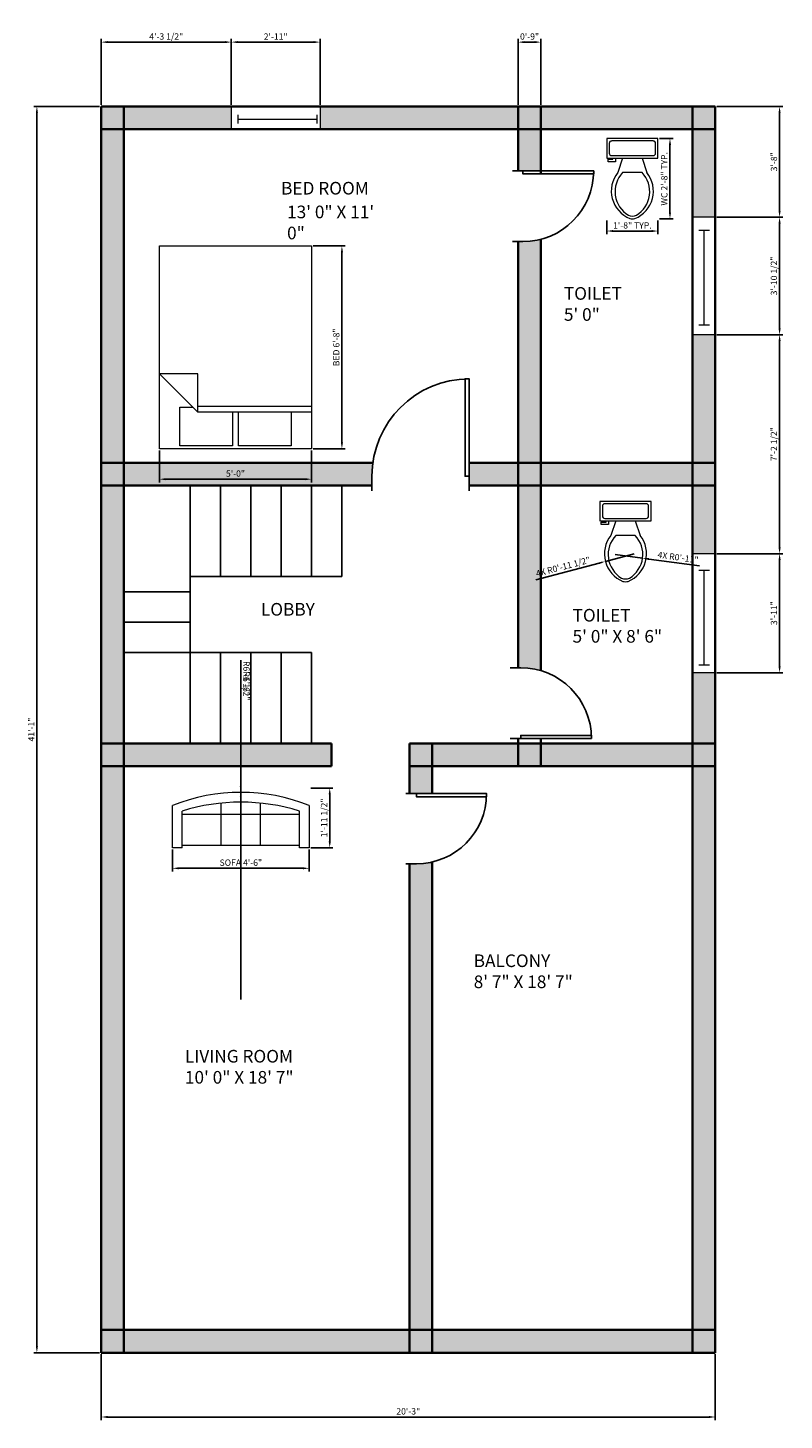
# Model space of a CAD drawing. Units: millimetres. Extents: x 2602 to 3574, y 848 to 1501.
# Tile 3 of 3: x 3274 to 3574, y 872 to 1423. Entities that reach past the tile are written whole.
import ezdxf

# ---------------------------------------------------------------- set-up
doc = ezdxf.new("R2010")
doc.units = ezdxf.units.MM
for name, color, linetype, lineweight in [('A-ANNO-DIMS', 170, 'Continuous', 18), ('A-AREA-IDEN', 200, 'Continuous', 18), ('A-FLOR-FIXT', 90, 'Continuous', 18), ('A-WALL-PATT', 140, 'Continuous', 13), ('doors', 10, 'Continuous', 25), ('furniture', 90, 'Continuous', 18), ('STAIRCASE', 30, 'Continuous', 25), ('walls', 140, 'Continuous', 35), ('windows', 40, 'Continuous', 18)]:
    doc.layers.add(name, color=color, linetype=linetype, lineweight=lineweight)
doc.styles.get("Standard").update_dxf_attribs({"font": 'arial.ttf'})
doc.dimstyles.new('ISO-25', dxfattribs={"dimtxt": 2.5, "dimasz": 2.5, "dimexe": 1.25, "dimexo": 0.625, "dimtad": 1, "dimdec": 0, "dimlunit": 3, "dimtxsty": 'Standard', "dimcen": 2.5, "dimadec": 0, "dimazin": 0, "dimtfac": 1, "dimtdec": 0, "dimtmove": 0, "dimatfit": 3, "dimfxl": 1, "dimarcsym": 0})

# ---------------------------------------------------------------- blocks, each defined once
blk = doc.blocks.new('*U2')
for p, q in [((0, 0), (0, -6)), ((40, 0), (40, -6))]:
    blk.add_line(p, q)
blk.add_lwpolyline([(0, 0), (0, 40), (1.75, 40), (1.75, 0)], close=True)
blk.add_arc((0, 0), 40, 0, 90)
blk = doc.blocks.new('*U23')
for p, q in [((0, 4), (0, 0)), ((0, 2), (36, 2)), ((36, 4), (36, 0))]:
    blk.add_line(p, q)
blk = doc.blocks.new('*U24')
for p, q in [((0, 4), (0, 0)), ((0, 2), (36, 2)), ((36, 4), (36, 0))]:
    blk.add_line(p, q)
blk = doc.blocks.new('Bed - Queen')
for p, q in [((0, -80.00003), (0, 0)), ((0, 0), (59.99999, 0)), ((59.99999, 0), (59.99999, -80.00003)), ((7.99999, -1.2), (28.79998, -1.2)), ((7.99999, -14.4), (7.99999, -1.2)), ((28.79998, -1.2), (28.79998, -14.4)), ((31.19999, -1.2), (51.99999, -1.2)), ((31.19999, -14.4), (31.19999, -1.2)), ((51.99999, -1.2), (51.99999, -16.4)), ((0, -14.4), (44.8, -14.4)), ((59.99999, -29.6), (44.8, -14.4)), ((44.8, -14.4), (44.8, -29.6)), ((51.99999, -16.4), (46.79936, -16.4)), ((44.8, -16.8), (0, -16.8)), ((44.8, -29.6), (59.99999, -29.6)), ((59.99999, -80.00003), (0, -80.00003))]:
    blk.add_line(p, q)
blk = doc.blocks.new('Sofa - Roundback 7 ft.')
for p, q in [((-12.00002, -32.4421), (-12.00003, -6.5971)), ((11.99997, -32.4421), (11.99998, -6.5971)), ((-36.000027, -34), (-36.000027, -11.4696)), ((-35.999844, -13.3819), (35.9998, -13.3819)), ((35.99998, -34), (35.99998, -11.4696)), ((-36.000027, -32.4421), (35.99998, -32.4421))]:
    blk.add_line(p, q)
for points in [[(-36.000027, -34), (-42.000027, -34), (-42.000027, -8)], [(41.99998, -8), (41.99998, -34), (35.99998, -34)]]:
    blk.add_lwpolyline(points)
for centre, radius, start, end in [((0, -114.25), 114.25, 68.43141, 111.5686), ((-0.00001, -127.1968), 121.1968, 72.72033, 107.2797)]:
    blk.add_arc(centre, radius, start, end)
blk = doc.blocks.new('Toilet - top')
for p, q in [((9.5, -6), (9.5, -2)), ((-10, -8.5), (-8, -8.5)), ((-10, -9.5), (-10, -8.5)), ((-7, -9.5), (-10, -9.5)), ((-8, -8.5), (-8, -8)), ((-7, -8), (-7, -9.5)), ((-4, -8), (-6, -14)), ((4, -8), (6, -14)), ((4, -14), (-4, -14))]:
    blk.add_line(p, q)
blk.add_lwpolyline([(10.5, -8), (10.5, 0), (-10.5, 0), (-10.5, -8)], close=True)
for points in [[(-9.5, -2), (-9.5, -6)], [(8.5, -1), (-8.5, -1)], [(-8.5, -7), (8.5, -7)]]:
    blk.add_lwpolyline(points)
for centre, radius, start, end in [((-8.62, -1.88), 0.884, 81.8699, 188.1301), ((8.62, -1.88), 0.884, 351.8699, 98.1301), ((-8.62, -6.12), 0.884, 171.8699, 278.1301), ((8.62, -6.12), 0.884, 261.8699, 8.1301), ((3.52, -21.58), 12.17, 141.4691, 247.9714), ((4.2, -21.82), 11.33, 136.3677, 238.9468), ((-3.52, -21.58), 12.17, 292.0284, 38.5307), ((-4.2, -21.82), 11.33, 301.053, 43.6321), ((0, -27.88), 4, 245.7318, 294.2682), ((0, -29), 4, 254.8605, 285.1395)]:
    blk.add_arc(centre, radius, start, end)
blk = doc.blocks.new('*D30')
at = {"layer": 'A-ANNO-DIMS', "color": 0, "lineweight": -2, "transparency": 16777216}
for p, q in [((3524.34, 1379.15), (3529.73, 1379.15)), ((3528.48, 1349.84), (3528.48, 1376.65)), ((3524.34, 1347.34), (3529.73, 1347.34))]:
    blk.add_line(p, q, dxfattribs=at)
at = {"layer": 'A-ANNO-DIMS', "color": 0, "transparency": 16777216}
for points in [[(3528.07, 1376.65), (3528.9, 1376.65), (3528.48, 1379.15)], [(3528.07, 1349.84), (3528.9, 1349.84), (3528.48, 1347.34)]]:
    blk.add_solid(points, dxfattribs=at)
at = {"layer": 'Defpoints', "color": 0, "transparency": 16777216}
for p in [(3523.71, 1379.15), (3528.48, 1379.15), (3523.71, 1347.34)]:
    blk.add_point(p, dxfattribs=at)
at = {"layer": 'A-ANNO-DIMS', "color": 0, "transparency": 16777216, "insert": (3526.56, 1363.24), "char_height": 2.5, "attachment_point": 5, "rotation": 90}
blk.add_mtext('WC 2\'-8" TYP.', dxfattribs=at)
blk = doc.blocks.new('*D31')
at = {"layer": 'A-ANNO-DIMS', "color": 0, "lineweight": -2, "transparency": 16777216}
for p, q in [((3503.49, 1346.71), (3503.49, 1341.31)), ((3523.71, 1346.71), (3523.71, 1341.31)), ((3505.99, 1342.56), (3521.21, 1342.56))]:
    blk.add_line(p, q, dxfattribs=at)
at = {"layer": 'A-ANNO-DIMS', "color": 0, "transparency": 16777216}
for points in [[(3505.99, 1342.98), (3505.99, 1342.15), (3503.49, 1342.56)], [(3521.21, 1342.98), (3521.21, 1342.15), (3523.71, 1342.56)]]:
    blk.add_solid(points, dxfattribs=at)
at = {"layer": 'Defpoints', "color": 0, "transparency": 16777216}
for p in [(3503.49, 1347.34), (3523.71, 1347.34), (3523.71, 1342.56)]:
    blk.add_point(p, dxfattribs=at)
at = {"layer": 'A-ANNO-DIMS', "color": 0, "transparency": 16777216, "insert": (3513.6, 1344.47), "char_height": 2.5, "attachment_point": 5}
blk.add_mtext('1\'-8" TYP.', dxfattribs=at)
blk = doc.blocks.new('*D34')
at = {"layer": 'A-ANNO-DIMS', "color": 0, "lineweight": -2, "transparency": 16777216}
for p, q in [((3387.25, 1336.66), (3399.91, 1336.66)), ((3398.66, 1334.16), (3398.66, 1258.93)), ((3387.25, 1256.43), (3399.91, 1256.43))]:
    blk.add_line(p, q, dxfattribs=at)
at = {"layer": 'A-ANNO-DIMS', "color": 0, "transparency": 16777216}
for points in [[(3398.25, 1334.16), (3399.08, 1334.16), (3398.66, 1336.66)], [(3398.25, 1258.93), (3399.08, 1258.93), (3398.66, 1256.43)]]:
    blk.add_solid(points, dxfattribs=at)
at = {"layer": 'Defpoints', "color": 0, "transparency": 16777216}
for p in [(3386.63, 1336.66), (3386.63, 1256.43), (3398.66, 1256.43)]:
    blk.add_point(p, dxfattribs=at)
at = {"layer": 'A-ANNO-DIMS', "color": 0, "transparency": 16777216, "insert": (3396.76, 1296.54), "char_height": 2.5, "attachment_point": 5, "rotation": 90}
blk.add_mtext('BED 6\'-8"', dxfattribs=at)
blk = doc.blocks.new('*D35')
at = {"layer": 'A-ANNO-DIMS', "color": 0, "lineweight": -2, "transparency": 16777216}
for p, q in [((3326.46, 1255.8), (3326.46, 1243.14)), ((3386.63, 1255.8), (3386.63, 1243.14)), ((3384.13, 1244.39), (3328.96, 1244.39))]:
    blk.add_line(p, q, dxfattribs=at)
at = {"layer": 'A-ANNO-DIMS', "color": 0, "transparency": 16777216}
for points in [[(3328.96, 1244.81), (3328.96, 1243.98), (3326.46, 1244.39)], [(3384.13, 1244.81), (3384.13, 1243.98), (3386.63, 1244.39)]]:
    blk.add_solid(points, dxfattribs=at)
at = {"layer": 'Defpoints', "color": 0, "transparency": 16777216}
for p in [(3326.46, 1256.43), (3386.63, 1256.43), (3326.46, 1244.39)]:
    blk.add_point(p, dxfattribs=at)
at = {"layer": 'A-ANNO-DIMS', "color": 0, "transparency": 16777216, "insert": (3356.54, 1246.29), "char_height": 2.5, "attachment_point": 5}
blk.add_mtext('5\'-0"', dxfattribs=at)
blk = doc.blocks.new('*D38')
at = {"layer": 'A-ANNO-DIMS', "color": 0, "lineweight": -2, "transparency": 16777216}
for p, q in [((3331.58, 1097.96), (3331.58, 1089.21)), ((3385.72, 1097.96), (3385.72, 1089.21)), ((3334.08, 1090.46), (3383.22, 1090.46))]:
    blk.add_line(p, q, dxfattribs=at)
at = {"layer": 'A-ANNO-DIMS', "color": 0, "transparency": 16777216}
for points in [[(3334.08, 1090.88), (3334.08, 1090.05), (3331.58, 1090.46)], [(3383.22, 1090.88), (3383.22, 1090.05), (3385.72, 1090.46)]]:
    blk.add_solid(points, dxfattribs=at)
at = {"layer": 'Defpoints', "color": 0, "transparency": 16777216}
for p in [(3331.58, 1098.59), (3385.72, 1098.59), (3385.72, 1090.46)]:
    blk.add_point(p, dxfattribs=at)
at = {"layer": 'A-ANNO-DIMS', "color": 0, "transparency": 16777216, "insert": (3358.65, 1092.38), "char_height": 2.5, "attachment_point": 5}
blk.add_mtext('SOFA 4\'-6"', dxfattribs=at)
blk = doc.blocks.new('*D39')
at = {"layer": 'A-ANNO-DIMS', "color": 0, "lineweight": -2, "transparency": 16777216}
for p, q in [((3386.34, 1122.22), (3395.09, 1122.22)), ((3393.84, 1101.09), (3393.84, 1119.72)), ((3386.34, 1098.59), (3395.09, 1098.59))]:
    blk.add_line(p, q, dxfattribs=at)
at = {"layer": 'A-ANNO-DIMS', "color": 0, "transparency": 16777216}
for points in [[(3393.42, 1119.72), (3394.26, 1119.72), (3393.84, 1122.22)], [(3393.42, 1101.09), (3394.26, 1101.09), (3393.84, 1098.59)]]:
    blk.add_solid(points, dxfattribs=at)
at = {"layer": 'Defpoints', "color": 0, "transparency": 16777216}
for p in [(3385.72, 1122.22), (3393.84, 1122.22), (3385.72, 1098.59)]:
    blk.add_point(p, dxfattribs=at)
at = {"layer": 'A-ANNO-DIMS', "color": 0, "transparency": 16777216, "insert": (3391.92, 1110.4), "char_height": 2.5, "attachment_point": 5, "rotation": 90}
blk.add_mtext('1\'-11 1/2"', dxfattribs=at)
blk = doc.blocks.new('*D48')
at = {"layer": 'A-ANNO-DIMS', "color": 0, "lineweight": -2, "transparency": 16777216}
for p, q in [((3303.41, 898.23), (3303.41, 872.15)), ((3546.41, 898.23), (3546.41, 872.15)), ((3305.91, 873.4), (3543.91, 873.4))]:
    blk.add_line(p, q, dxfattribs=at)
at = {"layer": 'A-ANNO-DIMS', "color": 0, "transparency": 16777216}
for points in [[(3305.91, 873.82), (3305.91, 872.99), (3303.41, 873.4)], [(3543.91, 873.82), (3543.91, 872.99), (3546.41, 873.4)]]:
    blk.add_solid(points, dxfattribs=at)
at = {"layer": 'Defpoints', "color": 0, "transparency": 16777216}
for p in [(3303.41, 898.85), (3546.41, 898.85), (3546.41, 873.4)]:
    blk.add_point(p, dxfattribs=at)
at = {"layer": 'A-ANNO-DIMS', "color": 0, "transparency": 16777216, "insert": (3424.91, 875.31), "char_height": 2.5, "attachment_point": 5}
blk.add_mtext('20\'-3"', dxfattribs=at)
blk = doc.blocks.new('*D49')
at = {"layer": 'A-ANNO-DIMS', "color": 0, "lineweight": -2, "transparency": 16777216}
for p, q in [((3302.78, 1391.85), (3276.71, 1391.85)), ((3277.96, 901.35), (3277.96, 1389.35)), ((3302.78, 898.85), (3276.71, 898.85))]:
    blk.add_line(p, q, dxfattribs=at)
at = {"layer": 'A-ANNO-DIMS', "color": 0, "transparency": 16777216}
for points in [[(3277.54, 1389.35), (3278.38, 1389.35), (3277.96, 1391.85)], [(3277.54, 901.35), (3278.38, 901.35), (3277.96, 898.85)]]:
    blk.add_solid(points, dxfattribs=at)
at = {"layer": 'Defpoints', "color": 0, "transparency": 16777216}
for p in [(3277.96, 1391.85), (3303.41, 1391.85), (3303.41, 898.85)]:
    blk.add_point(p, dxfattribs=at)
at = {"layer": 'A-ANNO-DIMS', "color": 0, "transparency": 16777216, "insert": (3276.08, 1145.35), "char_height": 2.5, "attachment_point": 5, "rotation": 90}
blk.add_mtext('41\'-1"', dxfattribs=at)
blk = doc.blocks.new('*D50')
at = {"layer": 'A-ANNO-DIMS', "color": 0, "lineweight": -2, "transparency": 16777216}
for p, q in [((3468.41, 1392.48), (3468.41, 1418.55)), ((3470.91, 1417.3), (3474.91, 1417.3)), ((3477.41, 1392.48), (3477.41, 1418.55))]:
    blk.add_line(p, q, dxfattribs=at)
at = {"layer": 'A-ANNO-DIMS', "color": 0, "transparency": 16777216}
for points in [[(3470.91, 1417.72), (3470.91, 1416.89), (3468.41, 1417.3)], [(3474.91, 1417.72), (3474.91, 1416.89), (3477.41, 1417.3)]]:
    blk.add_solid(points, dxfattribs=at)
at = {"layer": 'Defpoints', "color": 0, "transparency": 16777216}
for p in [(3477.41, 1417.3), (3468.41, 1391.85), (3477.41, 1391.85)]:
    blk.add_point(p, dxfattribs=at)
at = {"layer": 'A-ANNO-DIMS', "color": 0, "transparency": 16777216, "insert": (3472.91, 1419.2), "char_height": 2.5, "attachment_point": 5}
blk.add_mtext('0\'-9"', dxfattribs=at)
blk = doc.blocks.new('*D51')
at = {"layer": 'A-ANNO-DIMS', "color": 0, "lineweight": -2, "transparency": 16777216}
for p, q in [((3303.41, 1392.48), (3303.41, 1418.55)), ((3305.91, 1417.3), (3352.39, 1417.3)), ((3354.89, 1392.48), (3354.89, 1418.55))]:
    blk.add_line(p, q, dxfattribs=at)
at = {"layer": 'A-ANNO-DIMS', "color": 0, "transparency": 16777216}
for points in [[(3305.91, 1417.72), (3305.91, 1416.89), (3303.41, 1417.3)], [(3352.39, 1417.72), (3352.39, 1416.89), (3354.89, 1417.3)]]:
    blk.add_solid(points, dxfattribs=at)
at = {"layer": 'Defpoints', "color": 0, "transparency": 16777216}
for p in [(3354.89, 1417.3), (3303.41, 1391.85), (3354.89, 1391.85)]:
    blk.add_point(p, dxfattribs=at)
at = {"layer": 'A-ANNO-DIMS', "color": 0, "transparency": 16777216, "insert": (3329.15, 1419.22), "char_height": 2.5, "attachment_point": 5}
blk.add_mtext('4\'-3 1/2"', dxfattribs=at)
blk = doc.blocks.new('*D52')
at = {"layer": 'A-ANNO-DIMS', "color": 0, "lineweight": -2, "transparency": 16777216}
for p, q in [((3354.89, 1392.48), (3354.89, 1418.55)), ((3357.39, 1417.3), (3387.51, 1417.3)), ((3390.01, 1392.48), (3390.01, 1418.55))]:
    blk.add_line(p, q, dxfattribs=at)
at = {"layer": 'A-ANNO-DIMS', "color": 0, "transparency": 16777216}
for points in [[(3357.39, 1417.72), (3357.39, 1416.89), (3354.89, 1417.3)], [(3387.51, 1417.72), (3387.51, 1416.89), (3390.01, 1417.3)]]:
    blk.add_solid(points, dxfattribs=at)
at = {"layer": 'Defpoints', "color": 0, "transparency": 16777216}
for p in [(3390.01, 1417.3), (3354.89, 1391.85), (3390.01, 1391.85)]:
    blk.add_point(p, dxfattribs=at)
at = {"layer": 'A-ANNO-DIMS', "color": 0, "transparency": 16777216, "insert": (3372.45, 1419.18), "char_height": 2.5, "attachment_point": 5}
blk.add_mtext('2\'-11"', dxfattribs=at)
blk = doc.blocks.new('*D53')
at = {"layer": 'A-ANNO-DIMS', "color": 0, "lineweight": -2, "transparency": 16777216}
for p, q in [((3547.03, 1391.85), (3573.11, 1391.85)), ((3571.86, 1389.35), (3571.86, 1350.53)), ((3547.03, 1348.03), (3573.11, 1348.03))]:
    blk.add_line(p, q, dxfattribs=at)
at = {"layer": 'A-ANNO-DIMS', "color": 0, "transparency": 16777216}
for points in [[(3571.44, 1389.35), (3572.28, 1389.35), (3571.86, 1391.85)], [(3571.44, 1350.53), (3572.28, 1350.53), (3571.86, 1348.03)]]:
    blk.add_solid(points, dxfattribs=at)
at = {"layer": 'Defpoints', "color": 0, "transparency": 16777216}
for p in [(3546.41, 1391.85), (3546.41, 1348.03), (3571.86, 1348.03)]:
    blk.add_point(p, dxfattribs=at)
at = {"layer": 'A-ANNO-DIMS', "color": 0, "transparency": 16777216, "insert": (3569.96, 1369.94), "char_height": 2.5, "attachment_point": 5, "rotation": 90}
blk.add_mtext('3\'-8"', dxfattribs=at)
blk = doc.blocks.new('*D54')
at = {"layer": 'A-ANNO-DIMS', "color": 0, "lineweight": -2, "transparency": 16777216}
for p, q in [((3547.03, 1348.03), (3573.11, 1348.03)), ((3571.86, 1345.53), (3571.86, 1304.06)), ((3547.03, 1301.56), (3573.11, 1301.56))]:
    blk.add_line(p, q, dxfattribs=at)
at = {"layer": 'A-ANNO-DIMS', "color": 0, "transparency": 16777216}
for points in [[(3571.44, 1345.53), (3572.28, 1345.53), (3571.86, 1348.03)], [(3571.44, 1304.06), (3572.28, 1304.06), (3571.86, 1301.56)]]:
    blk.add_solid(points, dxfattribs=at)
at = {"layer": 'Defpoints', "color": 0, "transparency": 16777216}
for p in [(3546.41, 1348.03), (3546.41, 1301.56), (3571.86, 1301.56)]:
    blk.add_point(p, dxfattribs=at)
at = {"layer": 'A-ANNO-DIMS', "color": 0, "transparency": 16777216, "insert": (3569.94, 1324.79), "char_height": 2.5, "attachment_point": 5, "rotation": 90}
blk.add_mtext('3\'-10 1/2"', dxfattribs=at)
blk = doc.blocks.new('*D55')
at = {"layer": 'A-ANNO-DIMS', "color": 0, "lineweight": -2, "transparency": 16777216}
for p, q in [((3547.03, 1301.56), (3573.11, 1301.56)), ((3571.86, 1299.06), (3571.86, 1217.43)), ((3547.03, 1214.93), (3573.11, 1214.93))]:
    blk.add_line(p, q, dxfattribs=at)
at = {"layer": 'A-ANNO-DIMS', "color": 0, "transparency": 16777216}
for points in [[(3571.44, 1299.06), (3572.28, 1299.06), (3571.86, 1301.56)], [(3571.44, 1217.43), (3572.28, 1217.43), (3571.86, 1214.93)]]:
    blk.add_solid(points, dxfattribs=at)
at = {"layer": 'Defpoints', "color": 0, "transparency": 16777216}
for p in [(3546.41, 1301.56), (3546.41, 1214.93), (3571.86, 1214.93)]:
    blk.add_point(p, dxfattribs=at)
at = {"layer": 'A-ANNO-DIMS', "color": 0, "transparency": 16777216, "insert": (3569.94, 1258.24), "char_height": 2.5, "attachment_point": 5, "rotation": 90}
blk.add_mtext('7\'-2 1/2"', dxfattribs=at)
blk = doc.blocks.new('*D56')
at = {"layer": 'A-ANNO-DIMS', "color": 0, "lineweight": -2, "transparency": 16777216}
for p, q in [((3547.03, 1214.93), (3573.11, 1214.93)), ((3571.86, 1212.43), (3571.86, 1170.35)), ((3547.03, 1167.85), (3573.11, 1167.85))]:
    blk.add_line(p, q, dxfattribs=at)
at = {"layer": 'A-ANNO-DIMS', "color": 0, "transparency": 16777216}
for points in [[(3571.44, 1212.43), (3572.28, 1212.43), (3571.86, 1214.93)], [(3571.44, 1170.35), (3572.28, 1170.35), (3571.86, 1167.85)]]:
    blk.add_solid(points, dxfattribs=at)
at = {"layer": 'Defpoints', "color": 0, "transparency": 16777216}
for p in [(3546.41, 1214.93), (3546.41, 1167.85), (3571.86, 1167.85)]:
    blk.add_point(p, dxfattribs=at)
at = {"layer": 'A-ANNO-DIMS', "color": 0, "transparency": 16777216, "insert": (3569.96, 1191.39), "char_height": 2.5, "attachment_point": 5, "rotation": 90}
blk.add_mtext('3\'-11"', dxfattribs=at)
blk = doc.blocks.new('*D61')
at = {"layer": 'A-ANNO-DIMS', "color": 0, "lineweight": -2, "transparency": 16777216}
for p, q in [((3358.65, 1168.65), (3358.65, 1119.13)), ((3358.65, 1038.52), (3358.65, 1116.63))]:
    blk.add_line(p, q, dxfattribs=at)
at = {"layer": 'A-ANNO-DIMS', "color": 0, "transparency": 16777216}
blk.add_solid([(3359.06, 1119.13), (3358.23, 1119.13), (3358.65, 1116.63)], dxfattribs=at)
at = {"layer": 'Defpoints', "color": 0, "transparency": 16777216}
for p in [(3358.65, 1116.63), (3358.65, 1038.52)]:
    blk.add_point(p, dxfattribs=at)
at = {"layer": 'A-ANNO-DIMS', "color": 0, "transparency": 16777216, "insert": (3360.55, 1163.5), "char_height": 2.5, "attachment_point": 5, "rotation": 270.0001}
blk.add_mtext('R6\'-6"', dxfattribs=at)
blk = doc.blocks.new('*D62')
at = {"layer": 'A-ANNO-DIMS', "color": 0, "lineweight": -2, "transparency": 16777216}
for p, q in [((3358.65, 1172.74), (3358.65, 1123)), ((3358.65, 1046.86), (3358.65, 1120.5))]:
    blk.add_line(p, q, dxfattribs=at)
at = {"layer": 'A-ANNO-DIMS', "color": 0, "transparency": 16777216}
blk.add_solid([(3359.06, 1123), (3358.23, 1123), (3358.65, 1120.5)], dxfattribs=at)
at = {"layer": 'Defpoints', "color": 0, "transparency": 16777216}
for p in [(3358.65, 1120.5), (3358.65, 1046.86)]:
    blk.add_point(p, dxfattribs=at)
at = {"layer": 'A-ANNO-DIMS', "color": 0, "transparency": 16777216, "insert": (3360.57, 1164.68), "char_height": 2.5, "attachment_point": 5, "rotation": 270.0002}
blk.add_mtext('R6\'-1 1/2"', dxfattribs=at)
blk = doc.blocks.new('*D63')
at = {"layer": 'A-ANNO-DIMS', "color": 0, "lineweight": -2, "transparency": 16777216}
for p, q in [((3514.27, 1214.85), (3502.94, 1211.87)), ((3475.35, 1204.62), (3500.52, 1211.23))]:
    blk.add_line(p, q, dxfattribs=at)
at = {"layer": 'A-ANNO-DIMS', "color": 0, "transparency": 16777216}
blk.add_solid([(3500.42, 1211.64), (3500.63, 1210.83), (3502.94, 1211.87)], dxfattribs=at)
at = {"layer": 'Defpoints', "color": 0, "transparency": 16777216}
for p in [(3502.94, 1211.87), (3514.27, 1214.85)]:
    blk.add_point(p, dxfattribs=at)
at = {"layer": 'A-ANNO-DIMS', "color": 0, "transparency": 16777216, "insert": (3486.24, 1209.46), "char_height": 2.5, "attachment_point": 5, "rotation": 14.7202}
blk.add_mtext('4X R0\'-11 1/2"', dxfattribs=at)
blk = doc.blocks.new('*D64')
at = {"layer": 'A-ANNO-DIMS', "color": 0, "lineweight": -2, "transparency": 16777216}
for p, q in [((3506.84, 1214.62), (3517.65, 1213.15)), ((3540.14, 1210.08), (3520.12, 1212.81))]:
    blk.add_line(p, q, dxfattribs=at)
at = {"layer": 'A-ANNO-DIMS', "color": 0, "transparency": 16777216}
blk.add_solid([(3520.18, 1213.22), (3520.07, 1212.39), (3517.65, 1213.15)], dxfattribs=at)
at = {"layer": 'Defpoints', "color": 0, "transparency": 16777216}
for p in [(3506.84, 1214.62), (3517.65, 1213.15)]:
    blk.add_point(p, dxfattribs=at)
at = {"layer": 'A-ANNO-DIMS', "color": 0, "transparency": 16777216, "insert": (3531.63, 1213.16), "char_height": 2.5, "attachment_point": 5, "rotation": 352.2358}
blk.add_mtext('4X R0\'-11"', dxfattribs=at)

msp = doc.modelspace()

# ---------------------------------------------------------------- hatches: boundary and pattern name
at = {"layer": 'A-WALL-PATT'}
h = msp.add_hatch(color=256, dxfattribs=at)
h.dxf.hatch_style = 1
h.paths.add_polyline_path([(3312.41, 1382.85), (3303.41, 1382.85), (3303.41, 1250.85), (3312.41, 1250.85)])
h.paths.add_polyline_path([(3312.41, 1391.85), (3303.41, 1391.85), (3303.41, 1382.85), (3312.41, 1382.85)])
h.paths.add_polyline_path([(3354.89, 1391.85), (3312.41, 1391.85), (3312.41, 1382.85), (3354.89, 1382.85)])
h.paths.add_polyline_path([(3468.41, 1391.85), (3390.01, 1391.85), (3390.01, 1382.85), (3468.41, 1382.85)])
h.paths.add_polyline_path([(3477.41, 1391.85), (3468.41, 1391.85), (3468.41, 1382.85), (3477.41, 1382.85)])
h.paths.add_polyline_path([(3477.41, 1382.85), (3468.41, 1382.85), (3468.41, 1366.37), (3470.31, 1366.37), (3477.41, 1366.37)])
h.paths.add_polyline_path([(3537.41, 1391.85), (3477.41, 1391.85), (3477.41, 1382.85), (3537.41, 1382.85)])
h.paths.add_polyline_path([(3546.41, 1391.85), (3537.41, 1391.85), (3537.41, 1382.85), (3546.41, 1382.85)])
h.paths.add_polyline_path([(3546.41, 1382.85), (3537.41, 1382.85), (3537.41, 1348.03), (3546.41, 1348.03)])
h.paths.add_polyline_path([(3546.41, 1301.56), (3537.41, 1301.56), (3537.41, 1250.85), (3546.41, 1250.85)])
h.paths.add_polyline_path([(3477.41, 1339.31, -0.064198), (3470.31, 1338.39), (3468.41, 1338.39), (3468.41, 1250.85), (3477.41, 1250.85)])
h.paths.add_polyline_path([(3477.41, 1250.85), (3468.41, 1250.85), (3468.41, 1241.85), (3477.41, 1241.85)])
h.paths.add_polyline_path([(3537.41, 1250.85), (3477.41, 1250.85), (3477.41, 1241.85), (3537.41, 1241.85)])
h.paths.add_polyline_path([(3468.41, 1250.85), (3449.06, 1250.85), (3449.06, 1245.57), (3449.06, 1241.85), (3468.41, 1241.85)])
h.paths.add_polyline_path([(3546.41, 1250.85), (3537.41, 1250.85), (3537.41, 1241.85), (3546.41, 1241.85)])
h.paths.add_polyline_path([(3410.56, 1245.57, -0.034446), (3410.92, 1250.85), (3312.41, 1250.85), (3312.41, 1241.85), (3410.56, 1241.85)])
h.paths.add_polyline_path([(3312.41, 1250.85), (3303.41, 1250.85), (3303.41, 1241.85), (3312.41, 1241.85)])
h.paths.add_polyline_path([(3477.41, 1241.85), (3468.41, 1241.85), (3468.41, 1169.8), (3469.43, 1169.8, -0.0724), (3477.41, 1168.64)])
h.paths.add_polyline_path([(3546.41, 1241.85), (3537.41, 1241.85), (3537.41, 1214.93), (3546.41, 1214.93)])
h.paths.add_polyline_path([(3546.41, 1130.85), (3537.41, 1130.85), (3537.41, 907.85), (3546.41, 907.85)])
h.paths.add_polyline_path([(3546.41, 1139.85), (3537.41, 1139.85), (3537.41, 1130.85), (3546.41, 1130.85)])
h.paths.add_polyline_path([(3546.41, 1167.85), (3537.41, 1167.85), (3537.41, 1139.85), (3546.41, 1139.85)])
h.paths.add_polyline_path([(3537.41, 1139.85), (3477.41, 1139.85), (3477.41, 1130.85), (3537.41, 1130.85)])
h.paths.add_polyline_path([(3477.41, 1139.85), (3468.41, 1139.85), (3468.41, 1130.85), (3477.41, 1130.85)])
h.paths.add_polyline_path([(3468.41, 1139.85), (3434.41, 1139.85), (3434.41, 1130.85), (3468.41, 1130.85)])
h.paths.add_polyline_path([(3434.41, 1139.85), (3425.41, 1139.85), (3425.41, 1130.85), (3434.41, 1130.85)])
h.paths.add_polyline_path([(3434.41, 1130.85), (3425.41, 1130.85), (3425.41, 1120), (3428.15, 1120), (3434.41, 1120)])
h.paths.add_polyline_path([(3434.41, 1092.96, -0.056869), (3428.15, 1092.24), (3425.41, 1092.24), (3425.41, 907.85), (3434.41, 907.85)])
h.paths.add_polyline_path([(3312.41, 1130.85), (3303.41, 1130.85), (3303.41, 907.85), (3312.41, 907.85)])
h.paths.add_polyline_path([(3394.48, 1139.85), (3377.06, 1139.85), (3312.41, 1139.85), (3312.41, 1130.85), (3377.06, 1130.85), (3394.48, 1130.85)])
h.paths.add_polyline_path([(3312.41, 1241.85), (3303.41, 1241.85), (3303.41, 1139.85), (3312.41, 1139.85)])
h.paths.add_polyline_path([(3312.41, 1139.85), (3303.41, 1139.85), (3303.41, 1130.85), (3312.41, 1130.85)])
h.paths.add_polyline_path([(3312.41, 907.85), (3303.41, 907.85), (3303.41, 898.85), (3312.41, 898.85)])
h.paths.add_polyline_path([(3425.41, 907.85), (3312.41, 907.85), (3312.41, 898.85), (3425.41, 898.85)])
h.paths.add_polyline_path([(3537.41, 907.85), (3434.41, 907.85), (3434.41, 898.85), (3537.41, 898.85)])
h.paths.add_polyline_path([(3434.41, 907.85), (3425.41, 907.85), (3425.41, 898.85), (3434.41, 898.85)])
h.paths.add_polyline_path([(3546.41, 907.85), (3537.41, 907.85), (3537.41, 898.85), (3546.41, 898.85)])

# ---------------------------------------------------------------- linework, layer by layer
at = {"layer": 'STAIRCASE'}
for p, q in [((3338.57, 1241.85), (3338.57, 1139.85)), ((3350.57, 1241.85), (3350.57, 1205.85)), ((3350.57, 1241.85), (3350.57, 1205.85)), ((3362.57, 1241.85), (3362.57, 1205.85)), ((3362.57, 1241.85), (3362.57, 1205.85)), ((3374.57, 1241.85), (3374.57, 1205.85)), ((3374.57, 1241.85), (3374.57, 1205.85)), ((3386.57, 1241.85), (3386.57, 1205.85)), ((3386.57, 1241.85), (3386.57, 1205.85)), ((3398.57, 1241.85), (3398.57, 1205.85)), ((3398.57, 1205.85), (3338.57, 1205.85)), ((3338.57, 1199.85), (3312.41, 1199.85)), ((3338.57, 1187.85), (3312.41, 1187.85)), ((3367.08, 1175.85), (3312.41, 1175.85)), ((3386.57, 1175.85), (3331.54, 1175.85)), ((3350.57, 1175.85), (3350.57, 1139.85)), ((3362.57, 1175.85), (3362.57, 1139.85)), ((3374.57, 1175.85), (3374.57, 1139.85)), ((3386.57, 1175.85), (3386.57, 1139.85))]:
    msp.add_line(p, q, dxfattribs=at)
at = {"layer": 'walls'}
for p, q in [((3303.41, 1391.85), (3303.41, 898.85)), ((3303.41, 1391.85), (3546.41, 1391.85)), ((3312.41, 1391.85), (3312.41, 898.85)), ((3468.41, 1391.85), (3468.41, 1366.37)), ((3477.41, 1391.85), (3477.41, 1365.15)), ((3537.41, 1391.85), (3537.41, 898.85)), ((3546.41, 1391.85), (3546.41, 898.85)), ((3303.41, 1382.85), (3546.41, 1382.85)), ((3477.41, 1339.31), (3477.41, 1168.64)), ((3468.41, 1338.39), (3468.41, 1169.8)), ((3303.41, 1250.85), (3410.92, 1250.85)), ((3449.06, 1250.85), (3546.41, 1250.85)), ((3303.41, 1241.85), (3410.56, 1241.85)), ((3449.06, 1241.85), (3546.41, 1241.85)), ((3468.41, 1141.82), (3468.41, 1130.85)), ((3477.41, 1141.82), (3477.41, 1130.85)), ((3303.41, 1139.85), (3377.06, 1139.85)), ((3377.06, 1139.85), (3394.48, 1139.85)), ((3394.48, 1139.85), (3394.48, 1130.85)), ((3425.41, 1139.85), (3425.41, 1120)), ((3425.41, 1139.85), (3546.41, 1139.85)), ((3434.41, 1139.85), (3434.41, 1120)), ((3303.41, 1130.85), (3377.06, 1130.85)), ((3377.06, 1130.85), (3394.48, 1130.85)), ((3425.41, 1130.85), (3546.41, 1130.85)), ((3425.41, 1092.24), (3425.41, 898.85)), ((3434.41, 1092.96), (3434.41, 898.85)), ((3546.41, 907.85), (3303.41, 907.85)), ((3546.41, 898.85), (3303.41, 898.85))]:
    msp.add_line(p, q, dxfattribs=at)
at = {"layer": 'windows'}
for p, q in [((3354.89, 1391.85), (3354.89, 1382.85)), ((3390.01, 1391.85), (3390.01, 1382.85)), ((3546.41, 1348.03), (3537.41, 1348.03)), ((3546.41, 1301.56), (3537.41, 1301.56)), ((3546.41, 1214.93), (3537.41, 1214.93)), ((3546.41, 1214.93), (3546.41, 1214.93)), ((3546.41, 1167.85), (3537.41, 1167.85))]:
    msp.add_line(p, q, dxfattribs=at)

# ---------------------------------------------------------------- block references
at = {"layer": 'A-FLOR-FIXT', "xscale": 0.9626241279459772, "yscale": 0.9626241279459772, "zscale": 0.9626241279459772}
for p in [(3513.6, 1379.15), (3510.88, 1235.62)]:
    msp.add_blockref('Toilet - top', p, dxfattribs=at)
at = {"layer": 'doors', "rotation": 270}
for p, xscale, yscale, zscale in [((3470.31, 1366.37), 0.6994669211720895, 0.6994669211720895, 0.6994669211720895), ((3469.43, 1141.82), -0.6994669211720895, 0.6994669211720895, 0.6994669211720895), ((3428.15, 1120), 0.6939873961870512, 0.6939873961870512, 0.6939873961870512)]:
    msp.add_blockref('*U2', p, dxfattribs=dict(at, xscale=xscale, yscale=yscale, zscale=zscale))
at = {"layer": 'doors', "xscale": -0.9625884882041194, "yscale": 0.9625884882041194, "zscale": 0.9625884882041194}
msp.add_blockref('*U2', (3449.06, 1245.57), dxfattribs=at)
at = {"layer": 'furniture', "xscale": 1.002883941229482, "yscale": 1.002883941229482, "zscale": 1.002883941229482, "rotation": 180.0000000000001}
msp.add_blockref('Bed - Queen', (3386.63, 1256.43), dxfattribs=at)
at = {"layer": 'furniture', "xscale": 0.6445542439761325, "yscale": 0.6445542439761325, "zscale": 0.6445542439761325}
msp.add_blockref('Sofa - Roundback 7 ft.', (3358.65, 1120.5), dxfattribs=at)
at = {"layer": 'windows', "xscale": 0.8684296436834094, "yscale": 0.8684296436834094, "zscale": 0.8684296436834094}
msp.add_blockref('*U23', (3357.45, 1385.12), dxfattribs=at)
at = {"layer": 'windows', "xscale": 1.039543758085118, "yscale": 1.039543758085118, "zscale": 1.039543758085118, "rotation": 90}
for p in [(3544.12, 1305.45), (3544.1, 1170.94)]:
    msp.add_blockref('*U24', p, dxfattribs=at)

# ---------------------------------------------------------------- texts
at = {"layer": 'A-AREA-IDEN', "char_height": 5, "attachment_point": 1}
for s, width, insert in [('BED ROOM ', 40.4758, (3374.59, 1362.01)), ('13\' 0" X 11\' 0"', 36.0235, (3376.96, 1352.62)), ('TOILET \\P5\' 0"', 44.3884, (3486.5, 1320.39)), ('LOBBY', 41.4864, (3366.61, 1195.42)), ('TOILET\\P5\' 0" X 8\' 6"', 35.5939, (3489.94, 1193.07)), ('BALCONY\\P8\' 7" X 18\' 7"', 75.343, (3450.81, 1056.4)), ('LIVING ROOM \\P10\' 0" X 18\' 7"', 49.0971, (3336.53, 1018.62))]:
    msp.add_mtext_dynamic_manual_height_columns(s, width=width, gutter_width=12.5, heights=[0], dxfattribs=dict(at, insert=insert))

# ---------------------------------------------------------------- dimensions: what is measured, and where the dimension line sits
at = {"layer": 'A-ANNO-DIMS'}
for base, p1, p2, picture, middle in [((3354.89, 1417.3), (3303.41, 1391.85), (3354.89, 1391.85), '*D51', (3329.15, 1419.22)), ((3390.01, 1417.3), (3354.89, 1391.85), (3390.01, 1391.85), '*D52', (3372.45, 1419.18)), ((3477.41, 1417.3), (3468.41, 1391.85), (3477.41, 1391.85), '*D50', (3472.91, 1419.2)), ((3546.41, 873.4), (3303.41, 898.85), (3546.41, 898.85), '*D48', (3424.91, 875.31))]:
    dim = msp.add_linear_dim(base=base, p1=p1, p2=p2, dimstyle='ISO-25', override={"dimdec": 1, "dimlfac": 1, "dimrnd": 0, "dimzin": 1, "dimdsep": 46, "dimlunit": 4, "dimfrac": 2}, dxfattribs=at)
    dim.commit()
    dim.dimension.update_dxf_attribs({"geometry": picture, "text_midpoint": middle})
for base, p1, p2, angle, picture, middle in [((3277.96, 1391.85), (3303.41, 898.85), (3303.41, 1391.85), 90, '*D49', (3276.08, 1145.35)), ((3571.86, 1348.03), (3546.41, 1391.85), (3546.41, 1348.03), 90, '*D53', (3569.96, 1369.94)), ((3571.86, 1301.56), (3546.41, 1348.03), (3546.41, 1301.56), 90, '*D54', (3569.94, 1324.79)), ((3571.86, 1214.93), (3546.41, 1301.56), (3546.41, 1214.93), 90, '*D55', (3569.94, 1258.24)), ((3326.46, 1244.39), (3386.63, 1256.43), (3326.46, 1256.43), 180, '*D35', (3356.54, 1246.29)), ((3571.86, 1167.85), (3546.41, 1214.93), (3546.41, 1167.85), 90, '*D56', (3569.96, 1191.39)), ((3393.84, 1122.22), (3385.72, 1098.59), (3385.72, 1122.22), 90, '*D39', (3391.92, 1110.4))]:
    dim = msp.add_linear_dim(base=base, p1=p1, p2=p2, angle=angle, dimstyle='ISO-25', override={"dimdec": 1, "dimlfac": 1, "dimrnd": 0, "dimzin": 1, "dimdsep": 46, "dimlunit": 4, "dimfrac": 2}, dxfattribs=at)
    dim.commit()
    dim.dimension.update_dxf_attribs({"geometry": picture, "text_midpoint": middle})
for base, p1, p2, angle, text, picture, middle in [((3528.48, 1379.15), (3523.71, 1347.34), (3523.71, 1379.15), 90, 'WC <> TYP.', '*D30', (3526.56, 1363.24)), ((3398.66, 1256.43), (3386.63, 1336.66), (3386.63, 1256.43), 270, 'BED <>', '*D34', (3396.76, 1296.54))]:
    dim = msp.add_linear_dim(base=base, p1=p1, p2=p2, angle=angle, text=text, dimstyle='ISO-25', override={"dimdec": 1, "dimlfac": 1, "dimrnd": 0, "dimzin": 1, "dimdsep": 46, "dimlunit": 4, "dimfrac": 2}, dxfattribs=at)
    dim.commit()
    dim.dimension.update_dxf_attribs({"geometry": picture, "text_midpoint": middle})
for base, p1, p2, text, picture, middle in [((3523.71, 1342.56), (3503.49, 1347.34), (3523.71, 1347.34), '<> TYP.', '*D31', (3513.6, 1344.47)), ((3385.72, 1090.46), (3331.58, 1098.59), (3385.72, 1098.59), 'SOFA <>', '*D38', (3358.65, 1092.38))]:
    dim = msp.add_linear_dim(base=base, p1=p1, p2=p2, text=text, dimstyle='ISO-25', override={"dimdec": 1, "dimlfac": 1, "dimrnd": 0, "dimzin": 1, "dimdsep": 46, "dimlunit": 4, "dimfrac": 2}, dxfattribs=at)
    dim.commit()
    dim.dimension.update_dxf_attribs({"geometry": picture, "text_midpoint": middle})
for center, mpoint, picture, middle in [((3506.84, 1214.62), (3517.65, 1213.15), '*D64', (3531.63, 1213.16)), ((3514.27, 1214.85), (3502.94, 1211.87), '*D63', (3486.24, 1209.46))]:
    dim = msp.add_radius_dim(center=center, mpoint=mpoint, text='4X <>', dimstyle='ISO-25', override={"dimdec": 1, "dimlfac": 1, "dimrnd": 0, "dimzin": 1, "dimdsep": 46, "dimlunit": 4, "dimfrac": 2}, dxfattribs=at)
    dim.commit()
    dim.dimension.update_dxf_attribs({"geometry": picture, "text_midpoint": middle})
for center, mpoint, picture, middle in [((3358.65, 1046.86), (3358.65, 1120.5), '*D62', (3358.65, 1164.68)), ((3358.65, 1038.52), (3358.65, 1116.63), '*D61', (3358.65, 1163.5))]:
    dim = msp.add_radius_dim(center=center, mpoint=mpoint, dimstyle='ISO-25', override={"dimdec": 1, "dimlfac": 1, "dimrnd": 0, "dimzin": 1, "dimdsep": 46, "dimlunit": 4, "dimfrac": 2}, dxfattribs=at)
    dim.commit()
    dim.dimension.update_dxf_attribs({"geometry": picture, "text_midpoint": middle, "dimtype": 164})

doc.saveas('drawing.dxf')
